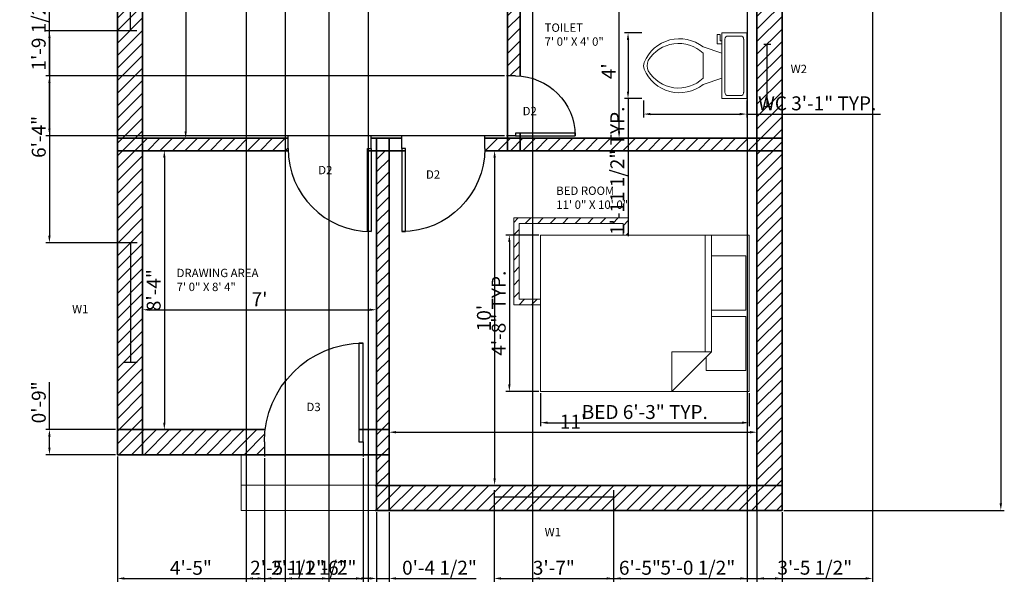
# Model space of a CAD drawing. Units: millimetres. Extents: x 2682 to 3042, y 1647 to 2164.
# Tile 1 of 4: x 2689 to 3042, y 1647 to 1852. Entities that reach past the tile are written whole.
import ezdxf

# ---------------------------------------------------------------- set-up
doc = ezdxf.new("R2010")
doc.units = ezdxf.units.MM
for name, color, linetype, lineweight in [('A-ANNO-TEXT', 170, 'Continuous', 18), ('A-AREA-IDEN', 170, 'Continuous', 18), ('A-FLOR-FIXT', 220, 'Continuous', 18), ('A-WALL-PATT', 3, 'Continuous', 13), ('dimensions', 140, 'Continuous', 18), ('doors', 40, 'Continuous', 25), ('furniture', 220, 'Continuous', 18), ('staircase', 10, 'Continuous', 18), ('walls', 70, 'Continuous', 35), ('windows', 50, 'Continuous', 25)]:
    doc.layers.add(name, color=color, linetype=linetype, lineweight=lineweight)
doc.layers.add('A-FURN-PATT', color=251, linetype='Continuous', lineweight=13, true_color=0x636466)
doc.styles.get("Standard").update_dxf_attribs({"font": 'arial.ttf'})
doc.dimstyles.new('ISO-25', dxfattribs={"dimtxt": 5, "dimasz": 2.5, "dimexe": 1.25, "dimexo": 0.625, "dimtad": 1, "dimdec": 0, "dimlunit": 3, "dimtxsty": 'Standard', "dimcen": 2.5, "dimadec": 0, "dimazin": 0, "dimtfac": 1, "dimtdec": 0, "dimtmove": 0, "dimatfit": 3, "dimfxl": 1, "dimarcsym": 0})

# ---------------------------------------------------------------- blocks, each defined once
blk = doc.blocks.new('*U2')
for p, q in [((0, 0), (0, -6)), ((40, 0), (40, -6))]:
    blk.add_line(p, q)
blk.add_lwpolyline([(0, 0), (0, 40), (1.75, 40), (1.75, 0)], close=True)
blk.add_arc((0, 0), 40, 0, 90)
blk = doc.blocks.new('*U4')
for p, q in [((0, 4), (0, 0)), ((36, 4), (36, 0)), ((0, 2), (36, 2))]:
    blk.add_line(p, q)
blk = doc.blocks.new('*U5')
for p, q in [((0, 4), (0, 0)), ((0, 2), (36, 2)), ((36, 4), (36, 0))]:
    blk.add_line(p, q)
blk = doc.blocks.new('Toilet - top')
for p, q in [((9.5, -6), (9.5, -2)), ((-10, -8.5), (-8, -8.5)), ((-10, -9.5), (-10, -8.5)), ((-8, -8.5), (-8, -8)), ((-7, -8), (-7, -9.5)), ((-4, -8), (-6, -14)), ((4, -8), (6, -14)), ((-7, -9.5), (-10, -9.5)), ((4, -14), (-4, -14))]:
    blk.add_line(p, q)
blk.add_lwpolyline([(10.5, -8), (10.5, 0), (-10.5, 0), (-10.5, -8)], close=True)
for points in [[(-9.5, -2), (-9.5, -6)], [(8.5, -1), (-8.5, -1)], [(-8.5, -7), (8.5, -7)]]:
    blk.add_lwpolyline(points)
for centre, radius, start, end in [((-8.62, -1.88), 0.884, 81.8699, 188.1301), ((8.62, -1.88), 0.884, 351.8699, 98.1301), ((-8.62, -6.12), 0.884, 171.8699, 278.1301), ((8.62, -6.12), 0.884, 261.8699, 8.1301), ((3.52, -21.58), 12.17, 141.4691, 247.9714), ((4.2, -21.82), 11.33, 136.3677, 238.9468), ((-3.52, -21.58), 12.17, 292.0284, 38.5307), ((-4.2, -21.82), 11.33, 301.053, 43.6321), ((0, -27.88), 4, 245.7318, 294.2682), ((0, -29), 4, 254.8605, 285.1395)]:
    blk.add_arc(centre, radius, start, end)
blk = doc.blocks.new('Bed - Queen')
for p, q in [((0, -80.00003), (0, 0)), ((0, 0), (59.99999, 0)), ((59.99999, 0), (59.99999, -80.00003)), ((7.99999, -1.2), (28.79998, -1.2)), ((7.99999, -14.4), (7.99999, -1.2)), ((28.79998, -1.2), (28.79998, -14.4)), ((31.19999, -1.2), (51.99999, -1.2)), ((31.19999, -14.4), (31.19999, -1.2)), ((51.99999, -1.2), (51.99999, -16.4)), ((0, -14.4), (44.8, -14.4)), ((59.99999, -29.6), (44.8, -14.4)), ((44.8, -14.4), (44.8, -29.6)), ((44.8, -16.8), (0, -16.8)), ((51.99999, -16.4), (46.79936, -16.4)), ((44.8, -29.6), (59.99999, -29.6)), ((59.99999, -80.00003), (0, -80.00003))]:
    blk.add_line(p, q)
blk = doc.blocks.new('*D20')
at = {"layer": 'Defpoints', "color": 0, "transparency": 16777216}
for p in [(2903.61, 1857.43), (2911.95, 1857.43), (2911.95, 1809.43)]:
    blk.add_point(p, dxfattribs=at)
at = {"layer": 'dimensions', "color": 0, "lineweight": -2, "transparency": 16777216}
for p, q in [((2911.33, 1857.43), (2902.36, 1857.43)), ((2903.61, 1811.93), (2903.61, 1854.93)), ((2911.33, 1809.43), (2902.36, 1809.43))]:
    blk.add_line(p, q, dxfattribs=at)
at = {"layer": 'dimensions', "color": 0, "transparency": 16777216}
for points in [[(2903.19, 1854.93), (2904.02, 1854.93), (2903.61, 1857.43)], [(2903.19, 1811.93), (2904.02, 1811.93), (2903.61, 1809.43)]]:
    blk.add_solid(points, dxfattribs=at)
at = {"layer": 'dimensions', "color": 0, "transparency": 16777216, "insert": (2900.48, 1833.43), "char_height": 5, "attachment_point": 5, "rotation": 90}
blk.add_mtext("4'", dxfattribs=at)
blk = doc.blocks.new('*D21')
at = {"layer": 'Defpoints', "color": 0, "transparency": 16777216}
for p in [(2953.09, 1703.98), (2821.09, 1700.9), (2953.09, 1700.9)]:
    blk.add_point(p, dxfattribs=at)
at = {"layer": 'dimensions', "color": 0, "lineweight": -2, "transparency": 16777216}
for p, q in [((2821.09, 1701.53), (2821.09, 1705.23)), ((2823.59, 1703.98), (2950.59, 1703.98)), ((2953.09, 1701.53), (2953.09, 1705.23))]:
    blk.add_line(p, q, dxfattribs=at)
at = {"layer": 'dimensions', "color": 0, "transparency": 16777216}
for points in [[(2823.59, 1704.4), (2823.59, 1703.57), (2821.09, 1703.98)], [(2950.59, 1704.4), (2950.59, 1703.57), (2953.09, 1703.98)]]:
    blk.add_solid(points, dxfattribs=at)
at = {"layer": 'dimensions', "color": 0, "transparency": 16777216, "insert": (2887.09, 1707.12), "char_height": 5, "attachment_point": 5}
blk.add_mtext("11'", dxfattribs=at)
blk = doc.blocks.new('*D22')
at = {"layer": 'Defpoints', "color": 0, "transparency": 16777216}
for p in [(2863.59, 1804.93), (2858.95, 1684.93), (2863.59, 1684.93)]:
    blk.add_point(p, dxfattribs=at)
at = {"layer": 'dimensions', "color": 0, "lineweight": -2, "transparency": 16777216}
for p, q in [((2862.96, 1804.93), (2857.7, 1804.93)), ((2858.95, 1802.43), (2858.95, 1687.43)), ((2862.96, 1684.93), (2857.7, 1684.93))]:
    blk.add_line(p, q, dxfattribs=at)
at = {"layer": 'dimensions', "color": 0, "transparency": 16777216}
for points in [[(2858.53, 1802.43), (2859.36, 1802.43), (2858.95, 1804.93)], [(2858.53, 1687.43), (2859.36, 1687.43), (2858.95, 1684.93)]]:
    blk.add_solid(points, dxfattribs=at)
at = {"layer": 'dimensions', "color": 0, "transparency": 16777216, "insert": (2855.77, 1744.93), "char_height": 5, "attachment_point": 5, "rotation": 90}
blk.add_mtext("10'", dxfattribs=at)
blk = doc.blocks.new('*D23')
at = {"layer": 'Defpoints', "color": 0, "transparency": 16777216}
for p in [(2816.59, 1747.9), (2732.59, 1743.81), (2816.59, 1743.81)]:
    blk.add_point(p, dxfattribs=at)
at = {"layer": 'dimensions', "color": 0, "lineweight": -2, "transparency": 16777216}
for p, q in [((2732.59, 1744.44), (2732.59, 1749.15)), ((2816.59, 1744.44), (2816.59, 1749.15)), ((2735.09, 1747.9), (2814.09, 1747.9))]:
    blk.add_line(p, q, dxfattribs=at)
at = {"layer": 'dimensions', "color": 0, "transparency": 16777216}
for points in [[(2735.09, 1748.32), (2735.09, 1747.49), (2732.59, 1747.9)], [(2814.09, 1748.32), (2814.09, 1747.49), (2816.59, 1747.9)]]:
    blk.add_solid(points, dxfattribs=at)
at = {"layer": 'dimensions', "color": 0, "transparency": 16777216, "insert": (2774.59, 1751.03), "char_height": 5, "attachment_point": 5}
blk.add_mtext("7'", dxfattribs=at)
blk = doc.blocks.new('*D24')
at = {"layer": 'Defpoints', "color": 0, "transparency": 16777216}
for p in [(2735.2, 1804.93), (2735.2, 1704.93), (2740.45, 1704.93)]:
    blk.add_point(p, dxfattribs=at)
at = {"layer": 'dimensions', "color": 0, "lineweight": -2, "transparency": 16777216}
for p, q in [((2735.83, 1804.93), (2741.7, 1804.93)), ((2740.45, 1802.43), (2740.45, 1707.43)), ((2735.83, 1704.93), (2741.7, 1704.93))]:
    blk.add_line(p, q, dxfattribs=at)
at = {"layer": 'dimensions', "color": 0, "transparency": 16777216}
for points in [[(2740.03, 1802.43), (2740.87, 1802.43), (2740.45, 1804.93)], [(2740.03, 1707.43), (2740.87, 1707.43), (2740.45, 1704.93)]]:
    blk.add_solid(points, dxfattribs=at)
at = {"layer": 'dimensions', "color": 0, "transparency": 16777216, "insert": (2737.27, 1754.93), "char_height": 5, "attachment_point": 5, "rotation": 90}
blk.add_mtext('8\'-4"', dxfattribs=at)
blk = doc.blocks.new('*D25')
at = {"layer": 'Defpoints', "color": 0, "transparency": 16777216}
for p in [(2751.08, 1998.43), (2748.1, 1809.43), (2751.08, 1809.43)]:
    blk.add_point(p, dxfattribs=at)
at = {"layer": 'dimensions', "color": 0, "lineweight": -2, "transparency": 16777216}
for p, q in [((2750.46, 1998.43), (2746.85, 1998.43)), ((2748.1, 1995.93), (2748.1, 1811.93)), ((2750.46, 1809.43), (2746.85, 1809.43))]:
    blk.add_line(p, q, dxfattribs=at)
at = {"layer": 'dimensions', "color": 0, "transparency": 16777216}
for points in [[(2747.68, 1995.93), (2748.52, 1995.93), (2748.1, 1998.43)], [(2747.68, 1811.93), (2748.52, 1811.93), (2748.1, 1809.43)]]:
    blk.add_solid(points, dxfattribs=at)
at = {"layer": 'dimensions', "color": 0, "transparency": 16777216, "insert": (2744.92, 1903.93), "char_height": 5, "attachment_point": 5, "rotation": 90}
blk.add_mtext('15\'-9"', dxfattribs=at)
blk = doc.blocks.new('*D27')
at = {"layer": 'Defpoints', "color": 0, "transparency": 16777216}
for p in [(2962.09, 2128.93), (2962.09, 1675.93), (3040.59, 1675.93)]:
    blk.add_point(p, dxfattribs=at)
at = {"layer": 'dimensions', "color": 0, "lineweight": -2, "transparency": 16777216}
for p, q in [((2962.71, 2128.93), (3041.84, 2128.93)), ((3040.59, 2126.43), (3040.59, 1678.43)), ((2962.71, 1675.93), (3041.84, 1675.93))]:
    blk.add_line(p, q, dxfattribs=at)
at = {"layer": 'dimensions', "color": 0, "transparency": 16777216}
for points in [[(3040.17, 2126.43), (3041, 2126.43), (3040.59, 2128.93)], [(3040.17, 1678.43), (3041, 1678.43), (3040.59, 1675.93)]]:
    blk.add_solid(points, dxfattribs=at)
at = {"layer": 'dimensions', "color": 0, "transparency": 16777216, "insert": (3037.41, 1902.43), "char_height": 5, "attachment_point": 5, "rotation": 90}
blk.add_mtext("38'", dxfattribs=at)
blk = doc.blocks.new('*D35')
at = {"layer": 'Defpoints', "color": 0, "transparency": 16777216}
for p in [(2875.45, 1718.62), (2950.23, 1718.62), (2950.23, 1707.4)]:
    blk.add_point(p, dxfattribs=at)
at = {"layer": 'dimensions', "color": 0, "lineweight": -2, "transparency": 16777216}
for p, q in [((2875.45, 1717.99), (2875.45, 1706.15)), ((2950.23, 1717.99), (2950.23, 1706.15)), ((2877.95, 1707.4), (2947.73, 1707.4))]:
    blk.add_line(p, q, dxfattribs=at)
at = {"layer": 'dimensions', "color": 0, "transparency": 16777216}
for points in [[(2877.95, 1707.82), (2877.95, 1706.98), (2875.45, 1707.4)], [(2947.73, 1707.82), (2947.73, 1706.98), (2950.23, 1707.4)]]:
    blk.add_solid(points, dxfattribs=at)
at = {"layer": 'dimensions', "color": 0, "transparency": 16777216, "insert": (2912.84, 1710.58), "char_height": 5, "attachment_point": 5}
blk.add_mtext('BED 6\'-3" TYP.', dxfattribs=at)
blk = doc.blocks.new('*D36')
at = {"layer": 'Defpoints', "color": 0, "transparency": 16777216}
for p in [(2875.45, 1774.7), (2864.24, 1718.62), (2875.45, 1718.62)]:
    blk.add_point(p, dxfattribs=at)
at = {"layer": 'dimensions', "color": 0, "lineweight": -2, "transparency": 16777216}
for p, q in [((2874.83, 1774.7), (2862.99, 1774.7)), ((2864.24, 1772.2), (2864.24, 1721.12)), ((2874.83, 1718.62), (2862.99, 1718.62))]:
    blk.add_line(p, q, dxfattribs=at)
at = {"layer": 'dimensions', "color": 0, "transparency": 16777216}
for points in [[(2863.82, 1772.2), (2864.66, 1772.2), (2864.24, 1774.7)], [(2863.82, 1721.12), (2864.66, 1721.12), (2864.24, 1718.62)]]:
    blk.add_solid(points, dxfattribs=at)
at = {"layer": 'dimensions', "color": 0, "transparency": 16777216, "insert": (2861.06, 1746.66), "char_height": 5, "attachment_point": 5, "rotation": 90}
blk.add_mtext('4\'-8" TYP.', dxfattribs=at)
blk = doc.blocks.new('*D37')
at = {"layer": 'Defpoints', "color": 0, "transparency": 16777216}
for p in [(2912.38, 1823.62), (2949.44, 1823.62), (2949.44, 1818.06)]:
    blk.add_point(p, dxfattribs=at)
at = {"layer": 'dimensions', "color": 0, "lineweight": -2, "transparency": 16777216}
for p, q in [((2912.38, 1822.99), (2912.38, 1816.81)), ((2949.44, 1822.99), (2949.44, 1816.81)), ((2914.88, 1818.06), (2946.94, 1818.06)), ((2949.44, 1818.06), (2997.45, 1818.06))]:
    blk.add_line(p, q, dxfattribs=at)
at = {"layer": 'dimensions', "color": 0, "transparency": 16777216}
for points in [[(2914.88, 1818.47), (2914.88, 1817.64), (2912.38, 1818.06)], [(2946.94, 1818.47), (2946.94, 1817.64), (2949.44, 1818.06)]]:
    blk.add_solid(points, dxfattribs=at)
at = {"layer": 'dimensions', "color": 0, "transparency": 16777216, "insert": (2974.7, 1821.27), "char_height": 5, "attachment_point": 5}
blk.add_mtext('WC 3\'-1" TYP.', dxfattribs=at)
blk = doc.blocks.new('*D38')
at = {"layer": 'Defpoints', "color": 0, "transparency": 16777216}
for p in [(2912.38, 1847.17), (2906.83, 1823.62), (2912.38, 1823.62)]:
    blk.add_point(p, dxfattribs=at)
at = {"layer": 'dimensions', "color": 0, "lineweight": -2, "transparency": 16777216}
for p, q in [((2911.76, 1847.17), (2905.58, 1847.17)), ((2906.83, 1844.67), (2906.83, 1826.12)), ((2911.76, 1823.62), (2905.58, 1823.62)), ((2906.83, 1823.62), (2906.83, 1774.32))]:
    blk.add_line(p, q, dxfattribs=at)
at = {"layer": 'dimensions', "color": 0, "transparency": 16777216}
for points in [[(2906.41, 1844.67), (2907.24, 1844.67), (2906.83, 1847.17)], [(2906.41, 1826.12), (2907.24, 1826.12), (2906.83, 1823.62)]]:
    blk.add_solid(points, dxfattribs=at)
at = {"layer": 'dimensions', "color": 0, "transparency": 16777216, "insert": (2903.62, 1797.72), "char_height": 5, "attachment_point": 5, "rotation": 90}
blk.add_mtext('1\'-11 1/2" TYP.', dxfattribs=at)
blk = doc.blocks.new('*D52')
at = {"layer": 'Defpoints', "color": 0, "transparency": 16777216}
for p in [(2769.81, 2100.93), (2799.51, 2100.93), (2799.51, 1651.55)]:
    blk.add_point(p, dxfattribs=at)
at = {"layer": 'dimensions', "color": 0, "lineweight": -2, "transparency": 16777216}
for p, q in [((2769.81, 2100.31), (2769.81, 1650.3)), ((2799.51, 2100.31), (2799.51, 1650.3)), ((2772.31, 1651.55), (2797.01, 1651.55))]:
    blk.add_line(p, q, dxfattribs=at)
at = {"layer": 'dimensions', "color": 0, "transparency": 16777216}
for points in [[(2772.31, 1651.97), (2772.31, 1651.13), (2769.81, 1651.55)], [(2797.01, 1651.97), (2797.01, 1651.13), (2799.51, 1651.55)]]:
    blk.add_solid(points, dxfattribs=at)
at = {"layer": 'dimensions', "color": 0, "transparency": 16777216, "insert": (2784.66, 1654.76), "char_height": 5, "attachment_point": 5}
blk.add_mtext('2\'-5 1/2"', dxfattribs=at)
blk = doc.blocks.new('*D54')
at = {"layer": 'Defpoints', "color": 0, "transparency": 16777216}
for p in [(2872.59, 1909.93), (2949.59, 1909.93), (2949.59, 1651.55)]:
    blk.add_point(p, dxfattribs=at)
at = {"layer": 'dimensions', "color": 0, "lineweight": -2, "transparency": 16777216}
for p, q in [((2872.59, 1909.3), (2872.59, 1650.3)), ((2949.59, 1909.3), (2949.59, 1650.3)), ((2875.09, 1651.55), (2947.09, 1651.55))]:
    blk.add_line(p, q, dxfattribs=at)
at = {"layer": 'dimensions', "color": 0, "transparency": 16777216}
for points in [[(2875.09, 1651.97), (2875.09, 1651.13), (2872.59, 1651.55)], [(2947.09, 1651.97), (2947.09, 1651.13), (2949.59, 1651.55)]]:
    blk.add_solid(points, dxfattribs=at)
at = {"layer": 'dimensions', "color": 0, "transparency": 16777216, "insert": (2911.09, 1654.73), "char_height": 5, "attachment_point": 5}
blk.add_mtext('6\'-5"', dxfattribs=at)
blk = doc.blocks.new('*D55')
at = {"layer": 'Defpoints', "color": 0, "transparency": 16777216}
for p in [(2953.09, 1902.43), (2994.59, 1861.93), (2994.59, 1651.55)]:
    blk.add_point(p, dxfattribs=at)
at = {"layer": 'dimensions', "color": 0, "lineweight": -2, "transparency": 16777216}
for p, q in [((2953.09, 1901.8), (2953.09, 1650.3)), ((2994.59, 1861.3), (2994.59, 1650.3)), ((2955.59, 1651.55), (2992.09, 1651.55))]:
    blk.add_line(p, q, dxfattribs=at)
at = {"layer": 'dimensions', "color": 0, "transparency": 16777216}
for points in [[(2955.59, 1651.97), (2955.59, 1651.13), (2953.09, 1651.55)], [(2992.09, 1651.97), (2992.09, 1651.13), (2994.59, 1651.55)]]:
    blk.add_solid(points, dxfattribs=at)
at = {"layer": 'dimensions', "color": 0, "transparency": 16777216, "insert": (2973.84, 1654.76), "char_height": 5, "attachment_point": 5}
blk.add_mtext('3\'-5 1/2"', dxfattribs=at)
blk = doc.blocks.new('*D56')
at = {"layer": 'Defpoints', "color": 0, "transparency": 16777216}
for p in [(2858.75, 1680.84), (2901.67, 1680.84), (2901.67, 1651.55)]:
    blk.add_point(p, dxfattribs=at)
at = {"layer": 'dimensions', "color": 0, "lineweight": -2, "transparency": 16777216}
for p, q in [((2858.75, 1680.21), (2858.75, 1650.3)), ((2901.67, 1680.21), (2901.67, 1650.3)), ((2861.25, 1651.55), (2899.17, 1651.55))]:
    blk.add_line(p, q, dxfattribs=at)
at = {"layer": 'dimensions', "color": 0, "transparency": 16777216}
for points in [[(2861.25, 1651.97), (2861.25, 1651.13), (2858.75, 1651.55)], [(2899.17, 1651.97), (2899.17, 1651.13), (2901.67, 1651.55)]]:
    blk.add_solid(points, dxfattribs=at)
at = {"layer": 'dimensions', "color": 0, "transparency": 16777216, "insert": (2880.21, 1654.73), "char_height": 5, "attachment_point": 5}
blk.add_mtext('3\'-7"', dxfattribs=at)
blk = doc.blocks.new('*D59')
at = {"layer": 'Defpoints', "color": 0, "transparency": 16777216}
for p in [(2783.8, 1996.99), (2813.59, 1996.99), (2813.59, 1651.55)]:
    blk.add_point(p, dxfattribs=at)
at = {"layer": 'dimensions', "color": 0, "lineweight": -2, "transparency": 16777216}
for p, q in [((2783.8, 1996.36), (2783.8, 1650.3)), ((2813.59, 1996.36), (2813.59, 1650.3)), ((2786.3, 1651.55), (2811.09, 1651.55))]:
    blk.add_line(p, q, dxfattribs=at)
at = {"layer": 'dimensions', "color": 0, "transparency": 16777216}
for points in [[(2786.3, 1651.97), (2786.3, 1651.13), (2783.8, 1651.55)], [(2811.09, 1651.97), (2811.09, 1651.13), (2813.59, 1651.55)]]:
    blk.add_solid(points, dxfattribs=at)
at = {"layer": 'dimensions', "color": 0, "transparency": 16777216, "insert": (2798.69, 1654.73), "char_height": 5, "attachment_point": 5}
blk.add_mtext('2\'-6"', dxfattribs=at)
blk = doc.blocks.new('*D60')
at = {"layer": 'Defpoints', "color": 0, "transparency": 16777216}
for p in [(2699.21, 1831.73), (2863.18, 1831.73), (2863.18, 1810.31)]:
    blk.add_point(p, dxfattribs=at)
at = {"layer": 'dimensions', "color": 0, "lineweight": -2, "transparency": 16777216}
for p, q in [((2699.21, 1831.73), (2699.21, 1859.95)), ((2862.55, 1831.73), (2697.96, 1831.73)), ((2699.21, 1812.81), (2699.21, 1829.23)), ((2862.55, 1810.31), (2697.96, 1810.31))]:
    blk.add_line(p, q, dxfattribs=at)
at = {"layer": 'dimensions', "color": 0, "transparency": 16777216}
for points in [[(2698.8, 1829.23), (2699.63, 1829.23), (2699.21, 1831.73)], [(2698.8, 1812.81), (2699.63, 1812.81), (2699.21, 1810.31)]]:
    blk.add_solid(points, dxfattribs=at)
at = {"layer": 'dimensions', "color": 0, "transparency": 16777216, "insert": (2696, 1847.09), "char_height": 5, "attachment_point": 5, "rotation": 90}
blk.add_mtext('1\'-9 1/2"', dxfattribs=at)
blk = doc.blocks.new('*D61')
at = {"layer": 'Defpoints', "color": 0, "transparency": 16777216}
for p in [(2776.38, 1695.25), (2811.76, 1695.25), (2811.76, 1651.55)]:
    blk.add_point(p, dxfattribs=at)
at = {"layer": 'dimensions', "color": 0, "lineweight": -2, "transparency": 16777216}
for p, q in [((2776.38, 1694.63), (2776.38, 1650.3)), ((2811.76, 1694.63), (2811.76, 1650.3)), ((2778.88, 1651.55), (2809.26, 1651.55))]:
    blk.add_line(p, q, dxfattribs=at)
at = {"layer": 'dimensions', "color": 0, "transparency": 16777216}
for points in [[(2778.88, 1651.97), (2778.88, 1651.13), (2776.38, 1651.55)], [(2809.26, 1651.97), (2809.26, 1651.13), (2811.76, 1651.55)]]:
    blk.add_solid(points, dxfattribs=at)
at = {"layer": 'dimensions', "color": 0, "transparency": 16777216, "insert": (2794.07, 1654.76), "char_height": 5, "attachment_point": 5}
blk.add_mtext('2\'-11 1/2"', dxfattribs=at)
blk = doc.blocks.new('*D62')
at = {"layer": 'Defpoints', "color": 0, "transparency": 16777216}
for p in [(2723.59, 1695.93), (2776.38, 1695.25), (2776.38, 1651.55)]:
    blk.add_point(p, dxfattribs=at)
at = {"layer": 'dimensions', "color": 0, "lineweight": -2, "transparency": 16777216}
for p, q in [((2723.59, 1695.3), (2723.59, 1650.3)), ((2776.38, 1694.63), (2776.38, 1650.3)), ((2726.09, 1651.55), (2773.88, 1651.55))]:
    blk.add_line(p, q, dxfattribs=at)
at = {"layer": 'dimensions', "color": 0, "transparency": 16777216}
for points in [[(2726.09, 1651.97), (2726.09, 1651.13), (2723.59, 1651.55)], [(2773.88, 1651.97), (2773.88, 1651.13), (2776.38, 1651.55)]]:
    blk.add_solid(points, dxfattribs=at)
at = {"layer": 'dimensions', "color": 0, "transparency": 16777216, "insert": (2749.98, 1654.72), "char_height": 5, "attachment_point": 5}
blk.add_mtext('4\'-5"', dxfattribs=at)
blk = doc.blocks.new('*D63')
at = {"layer": 'Defpoints', "color": 0, "transparency": 16777216}
for p in [(2699.21, 1704.93), (2723.59, 1704.93), (2723.59, 1695.93)]:
    blk.add_point(p, dxfattribs=at)
at = {"layer": 'dimensions', "color": 0, "lineweight": -2, "transparency": 16777216}
for p, q in [((2699.21, 1704.93), (2699.21, 1721.97)), ((2722.96, 1704.93), (2697.96, 1704.93)), ((2699.21, 1698.43), (2699.21, 1702.43)), ((2722.96, 1695.93), (2697.96, 1695.93))]:
    blk.add_line(p, q, dxfattribs=at)
at = {"layer": 'dimensions', "color": 0, "transparency": 16777216}
for points in [[(2698.8, 1702.43), (2699.63, 1702.43), (2699.21, 1704.93)], [(2698.8, 1698.43), (2699.63, 1698.43), (2699.21, 1695.93)]]:
    blk.add_solid(points, dxfattribs=at)
at = {"layer": 'dimensions', "color": 0, "transparency": 16777216, "insert": (2696.03, 1714.7), "char_height": 5, "attachment_point": 5, "rotation": 90}
blk.add_mtext('0\'-9"', dxfattribs=at)
blk = doc.blocks.new('*D64')
at = {"layer": 'Defpoints', "color": 0, "transparency": 16777216}
for p in [(2816.59, 1675.93), (2821.09, 1675.93), (2821.09, 1651.55)]:
    blk.add_point(p, dxfattribs=at)
at = {"layer": 'dimensions', "color": 0, "lineweight": -2, "transparency": 16777216}
for p, q in [((2816.59, 1675.3), (2816.59, 1650.3)), ((2821.09, 1675.3), (2821.09, 1650.3)), ((2814.09, 1651.55), (2811.59, 1651.55)), ((2816.59, 1651.55), (2821.09, 1651.55)), ((2823.59, 1651.55), (2852.28, 1651.55))]:
    blk.add_line(p, q, dxfattribs=at)
at = {"layer": 'dimensions', "color": 0, "transparency": 16777216}
for points in [[(2814.09, 1651.97), (2814.09, 1651.13), (2816.59, 1651.55)], [(2823.59, 1651.97), (2823.59, 1651.13), (2821.09, 1651.55)]]:
    blk.add_solid(points, dxfattribs=at)
at = {"layer": 'dimensions', "color": 0, "transparency": 16777216, "insert": (2839.18, 1654.76), "char_height": 5, "attachment_point": 5}
blk.add_mtext('0\'-4 1/2"', dxfattribs=at)
blk = doc.blocks.new('*D70')
at = {"layer": 'Defpoints', "color": 0, "transparency": 16777216}
for p in [(2728.2, 1847.86), (2699.21, 1771.91), (2728.36, 1771.91)]:
    blk.add_point(p, dxfattribs=at)
at = {"layer": 'dimensions', "color": 0, "lineweight": -2, "transparency": 16777216}
for p, q in [((2727.58, 1847.86), (2697.96, 1847.86)), ((2699.21, 1845.36), (2699.21, 1774.41)), ((2727.73, 1771.91), (2697.96, 1771.91))]:
    blk.add_line(p, q, dxfattribs=at)
at = {"layer": 'dimensions', "color": 0, "transparency": 16777216}
for points in [[(2698.8, 1845.36), (2699.63, 1845.36), (2699.21, 1847.86)], [(2698.8, 1774.41), (2699.63, 1774.41), (2699.21, 1771.91)]]:
    blk.add_solid(points, dxfattribs=at)
at = {"layer": 'dimensions', "color": 0, "transparency": 16777216, "insert": (2696.03, 1809.88), "char_height": 5, "attachment_point": 5, "rotation": 90}
blk.add_mtext('6\'-4"', dxfattribs=at)
blk = doc.blocks.new('*D71')
at = {"layer": 'Defpoints', "color": 0, "transparency": 16777216}
for p in [(2901.67, 1680.84), (2962.09, 1675.93), (2962.09, 1651.55)]:
    blk.add_point(p, dxfattribs=at)
at = {"layer": 'dimensions', "color": 0, "lineweight": -2, "transparency": 16777216}
for p, q in [((2901.67, 1680.21), (2901.67, 1650.3)), ((2962.09, 1675.3), (2962.09, 1650.3)), ((2904.17, 1651.55), (2959.59, 1651.55))]:
    blk.add_line(p, q, dxfattribs=at)
at = {"layer": 'dimensions', "color": 0, "transparency": 16777216}
for points in [[(2904.17, 1651.97), (2904.17, 1651.13), (2901.67, 1651.55)], [(2959.59, 1651.97), (2959.59, 1651.13), (2962.09, 1651.55)]]:
    blk.add_solid(points, dxfattribs=at)
at = {"layer": 'dimensions', "color": 0, "transparency": 16777216, "insert": (2931.88, 1654.76), "char_height": 5, "attachment_point": 5}
blk.add_mtext('5\'-0 1/2"', dxfattribs=at)

msp = doc.modelspace()

# ---------------------------------------------------------------- hatches: boundary and pattern name
at = {"layer": 'A-FURN-PATT'}
h = msp.add_hatch(dxfattribs=at)
h.set_pattern_fill('ANSI31', color=256)
h.paths.add_polyline_path([(2868.36, 2054.1), (2875.35, 2054.1), (2875.35, 2056.1), (2866.36, 2056.1), (2866.36, 2017.68), (2900.8, 2017.68), (2900.8, 2036.29), (2898.8, 2036.29), (2898.8, 2019.68), (2868.36, 2019.68)])
h.paths.add_polyline_path([(2907.02, 1780.81), (2865.81, 1780.81), (2865.81, 1749.67), (2875.45, 1749.67), (2875.45, 1751.67), (2867.81, 1751.67), (2867.81, 1778.81), (2905.02, 1778.81), (2905.02, 1774.7), (2907.02, 1774.7)])
at = {"layer": 'A-WALL-PATT'}
h = msp.add_hatch(dxfattribs=at)
h.set_pattern_fill('ANSI31', color=256)
h.paths.add_polyline_path([(2816.59, 2128.93), (2732.59, 2128.93), (2732.59, 2119.93), (2816.59, 2119.93)])
h.paths.add_polyline_path([(2953.09, 2128.93), (2821.09, 2128.93), (2821.09, 2119.93), (2953.09, 2119.93)])
h.paths.add_polyline_path([(2821.09, 2119.93), (2816.59, 2119.93), (2816.59, 2002.93), (2821.09, 2002.93)])
h.paths.add_polyline_path([(2821.09, 2128.93), (2816.59, 2128.93), (2816.59, 2119.93), (2821.09, 2119.93)])
h.paths.add_polyline_path([(2732.59, 2119.93), (2723.59, 2119.93), (2723.59, 2002.93), (2732.59, 2002.93)])
h.paths.add_polyline_path([(2732.59, 2128.93), (2723.59, 2128.93), (2723.59, 2119.93), (2732.59, 2119.93)])
h.paths.add_polyline_path([(2962.09, 2119.93), (2953.09, 2119.93), (2953.09, 2002.93), (2962.09, 2002.93)])
h.paths.add_polyline_path([(2962.09, 2128.93), (2953.09, 2128.93), (2953.09, 2119.93), (2962.09, 2119.93)])
h.paths.add_polyline_path([(2953.09, 2002.93), (2897.45, 2002.93), (2897.45, 2000.43, -0.023466), (2897.35, 1998.43), (2953.09, 1998.43)])
h.paths.add_polyline_path([(2962.09, 1998.43), (2953.09, 1998.43), (2953.09, 1950.43), (2962.09, 1950.43)])
h.paths.add_polyline_path([(2953.09, 1950.43), (2868.09, 1950.43), (2868.09, 1945.93), (2953.09, 1945.93)])
h.paths.add_polyline_path([(2994.59, 1950.43), (2962.09, 1950.43), (2962.09, 1945.93), (2994.59, 1945.93)])
h.paths.add_polyline_path([(2868.09, 1998.43), (2863.59, 1998.43), (2863.59, 1950.43), (2868.09, 1950.43)])
h.paths.add_polyline_path([(2868.09, 2002.93), (2863.59, 2002.93), (2863.59, 1998.43), (2868.09, 1998.43)])
h.paths.add_polyline_path([(2863.59, 2002.93), (2853.46, 2002.93, -0.011786), (2853.49, 2001.52), (2853.49, 1998.43), (2863.59, 1998.43)])
h.paths.add_polyline_path([(2783.8, 2001.45, -0.012351), (2783.84, 2002.93), (2756.59, 2002.93), (2756.59, 2002.69), (2732.59, 2002.93), (2732.59, 1998.43), (2783.8, 1998.43)])
h.paths.add_polyline_path([(2732.59, 2002.93), (2723.59, 2002.93), (2723.59, 1998.43), (2732.59, 1998.43)])
h.paths.add_polyline_path([(2732.59, 1998.43), (2723.59, 1998.43), (2723.59, 1809.43), (2732.59, 1809.43)])
h.paths.add_polyline_path([(2994.59, 1861.93), (2962.09, 1861.93), (2962.09, 1857.43), (2994.59, 1857.43)])
h.paths.add_polyline_path([(2999.09, 1884.37), (2994.59, 1884.37), (2994.59, 1861.93), (2999.09, 1861.93)])
h.paths.add_polyline_path([(2953.09, 1861.93), (2868.09, 1861.93), (2868.09, 1857.43), (2953.09, 1857.43)])
h.paths.add_polyline_path([(2962.09, 1861.93), (2953.09, 1861.93), (2953.09, 1857.43), (2962.09, 1857.43)])
h.paths.add_polyline_path([(2868.09, 1857.43), (2863.59, 1857.43), (2863.59, 1831.73), (2866.39, 1831.73, -0.019816), (2868.09, 1831.66)])
h.paths.add_polyline_path([(2868.09, 1861.93), (2863.59, 1861.93), (2863.59, 1857.43), (2868.09, 1857.43)])
h.paths.add_polyline_path([(2962.09, 1804.93), (2953.09, 1804.93), (2953.09, 1684.93), (2962.09, 1684.93)])
h.paths.add_polyline_path([(2962.09, 1857.43), (2953.09, 1857.43), (2953.09, 1809.43), (2962.09, 1809.43)])
h.paths.add_polyline_path([(2962.09, 1809.43), (2953.09, 1809.43), (2953.09, 1804.93), (2962.09, 1804.93)])
h.paths.add_polyline_path([(2953.09, 1809.43), (2868.09, 1809.43), (2868.09, 1804.93), (2953.09, 1804.93)])
h.paths.add_polyline_path([(2868.09, 1809.43), (2863.59, 1809.43), (2863.59, 1804.93), (2868.09, 1804.93)])
h.paths.add_polyline_path([(2863.59, 1809.43), (2855.42, 1809.43), (2855.42, 1805.73, -0.006742), (2855.41, 1804.93), (2863.59, 1804.93)])
h.paths.add_polyline_path([(2953.09, 1684.93), (2863.59, 1684.93), (2821.09, 1684.93), (2821.09, 1675.93), (2863.59, 1675.93), (2953.09, 1675.93)])
h.paths.add_polyline_path([(2962.09, 1684.93), (2953.09, 1684.93), (2953.09, 1675.93), (2962.09, 1675.93)])
h.paths.add_polyline_path([(2821.09, 1804.93), (2816.59, 1804.93), (2816.59, 1704.93), (2821.09, 1704.93)])
h.paths.add_polyline_path([(2821.09, 1695.93), (2816.59, 1695.93), (2816.59, 1684.93), (2821.09, 1684.93)])
h.paths.add_polyline_path([(2821.09, 1704.93), (2816.59, 1704.93), (2816.59, 1695.93), (2821.09, 1695.93)])
h.paths.add_polyline_path([(2821.09, 1684.93), (2816.59, 1684.93), (2816.59, 1675.93), (2821.09, 1675.93)])
h.paths.add_polyline_path([(2776.38, 1700.56, -0.030957), (2776.65, 1704.93), (2732.59, 1704.93), (2732.59, 1695.93), (2776.38, 1695.93)])
h.paths.add_polyline_path([(2732.59, 1804.93), (2723.59, 1804.93), (2723.59, 1704.93), (2732.59, 1704.93)])
h.paths.add_polyline_path([(2732.59, 1704.93), (2723.59, 1704.93), (2723.59, 1695.93), (2732.59, 1695.93)])
h.paths.add_polyline_path([(2999.09, 1945.93), (2994.59, 1945.93), (2994.59, 1937.59), (2999.09, 1937.59)])
h.paths.add_polyline_path([(2999.09, 1937.59), (2996.77, 1937.59), (2996.77, 1884.37), (2999.09, 1884.37)])
h.paths.add_polyline_path([(2996.77, 1937.59), (2994.59, 1937.59), (2994.59, 1884.37), (2996.77, 1884.37)])
h.paths.add_polyline_path([(2784.83, 1809.43), (2732.59, 1809.43), (2732.59, 1804.93), (2784.84, 1804.93, -0.006742), (2784.83, 1805.73)])
h.paths.add_polyline_path([(2732.59, 1809.43), (2723.59, 1809.43), (2723.59, 1804.93), (2732.59, 1804.93)])

# ---------------------------------------------------------------- linework, layer by layer
at = {"layer": 'furniture'}
for points in [[(2875.45, 1749.67), (2865.81, 1749.67), (2865.81, 1780.81), (2907.02, 1780.81), (2907.02, 1774.7)], [(2875.45, 1751.67), (2867.81, 1751.67), (2867.81, 1778.81), (2905.02, 1778.81), (2905.02, 1774.7)]]:
    msp.add_lwpolyline(points, dxfattribs=at)
at = {"layer": 'staircase'}
for p, q in [((2768.01, 1695.93), (2768.01, 1684.96)), ((2768.01, 1684.96), (2816.59, 1684.96)), ((2768.01, 1684.96), (2768.01, 1678.16)), ((2768.01, 1675.93), (2768.01, 1678.16)), ((2768.01, 1675.93), (2816.59, 1675.93)), ((2816.59, 1675.93), (2768.01, 1675.93))]:
    msp.add_line(p, q, dxfattribs=at)
at = {"layer": 'walls'}
for p, q in [((2723.59, 2128.93), (2723.59, 1695.93)), ((2732.59, 2128.93), (2732.59, 1695.93)), ((2953.09, 2128.93), (2953.09, 1675.93)), ((2863.59, 1861.93), (2863.59, 1804.93)), ((2868.09, 1861.93), (2868.09, 1831.66)), ((2962.09, 1861.93), (2962.09, 1675.93)), ((2723.59, 1809.43), (2784.83, 1809.43)), ((2814.62, 1809.43), (2825.64, 1809.43)), ((2816.59, 1809.43), (2816.59, 1675.93)), ((2821.09, 1809.43), (2821.09, 1695.93)), ((2821.09, 1809.43), (2821.09, 1675.93)), ((2855.42, 1809.43), (2868.09, 1809.43)), ((2863.59, 1809.43), (2962.09, 1809.43)), ((2868.09, 1811.25), (2868.09, 1804.93)), ((2723.59, 1804.93), (2784.84, 1804.93)), ((2813.32, 1804.93), (2826.94, 1804.93)), ((2855.41, 1804.93), (2868.09, 1804.93)), ((2863.59, 1804.93), (2962.09, 1804.93)), ((2723.59, 1704.93), (2776.65, 1704.93)), ((2810.21, 1704.93), (2821.09, 1704.93)), ((2723.59, 1695.93), (2821.09, 1695.93)), ((2863.59, 1684.93), (2816.06, 1684.93)), ((2863.59, 1684.93), (2962.09, 1684.93)), ((2863.59, 1675.93), (2816.06, 1675.93)), ((2863.59, 1675.93), (2962.09, 1675.93))]:
    msp.add_line(p, q, dxfattribs=at)

# ---------------------------------------------------------------- block references
at = {"layer": 'A-FLOR-FIXT', "xscale": 1.121371250506495, "yscale": 1.121371250506495, "zscale": 1.121371250506495, "rotation": 269.9999999999973}
msp.add_blockref('Toilet - top', (2949.44, 1835.39), dxfattribs=at)
at = {"layer": 'doors'}
for p, xscale, yscale, zscale, rotation in [((2866.39, 1810.31), -0.5354065160128529, 0.5354065160128529, 0.5354065160128529, 270), ((2814.62, 1805.73), 0.744697270728857, 0.744697270728857, 0.744697270728857, 180), ((2825.64, 1805.73), -0.744697270728857, 0.744697270728857, 0.744697270728857, 180)]:
    msp.add_blockref('*U2', p, dxfattribs=dict(at, xscale=xscale, yscale=yscale, zscale=zscale, rotation=rotation))
at = {"layer": 'doors', "xscale": -0.8844760457410782, "yscale": 0.8844760457410782, "zscale": 0.8844760457410782}
msp.add_blockref('*U2', (2811.76, 1700.56), dxfattribs=at)
at = {"layer": 'furniture', "xscale": 0.9346925861226617, "yscale": 0.9346925861226617, "zscale": 0.9346925861226617, "rotation": 269.9999999999884}
msp.add_blockref('Bed - Queen', (2950.23, 1774.7), dxfattribs=at)
at = {"layer": 'windows'}
for name, p, xscale, yscale, zscale, rotation in [('*U4', (2725.82, 1890.78), 1.192221816707046, 1.192221816707046, 1.192221816707046, 270), ('*U5', (2958.03, 1820.84), 0.6208711624712905, 0.6208711624712905, 0.6208711624712905, 90), ('*U4', (2725.97, 1771.91), 1.192221816707046, 1.192221816707046, 1.192221816707046, 270)]:
    msp.add_blockref(name, p, dxfattribs=dict(at, xscale=xscale, yscale=yscale, zscale=zscale, rotation=rotation))
at = {"layer": 'windows', "xscale": 1.192221816707046, "yscale": 1.192221816707046, "zscale": 1.192221816707046}
msp.add_blockref('*U4', (2858.75, 1678.45), dxfattribs=at)

# ---------------------------------------------------------------- texts
at = {"layer": 'A-ANNO-TEXT', "char_height": 3, "attachment_point": 1}
for s, width, insert in [('W2', 17.3612, (2965.17, 1835.74)), ('D2', 10.4757, (2869.01, 1820.65)), ('D2', 15.5328, (2795.66, 1799.48)), ('D2', 14.1591, (2834.33, 1797.89)), ('W1', 12.3833, (2707.35, 1749.66)), ('D3', 15.4098, (2791.46, 1714.55)), ('W1', 13.8484, (2876.9, 1669.69))]:
    msp.add_mtext_dynamic_manual_height_columns(s, width=width, gutter_width=12.5, heights=[0], dxfattribs=dict(at, insert=insert))
at = {"layer": 'A-AREA-IDEN', "char_height": 3, "attachment_point": 1}
for s, width, insert in [('TOILET\\P7\' 0" X 4\' 0"', 39.5175, (2876.89, 1850.56)), ('BED ROOM \\P11\' 0" X 10\' 0"', 47.2752, (2881.07, 1792.08)), ('DRAWING AREA \\P7\' 0" X 8\' 4"', 55.9803, (2744.85, 1762.59))]:
    msp.add_mtext_dynamic_manual_height_columns(s, width=width, gutter_width=12.5, heights=[0], dxfattribs=dict(at, insert=insert))

# ---------------------------------------------------------------- dimensions: what is measured, and where the dimension line sits
at = {"layer": 'dimensions'}
for base, p1, p2, angle, text, override, picture, middle in [((3040.59, 1675.93), (2962.09, 2128.93), (2962.09, 1675.93), 90, "38'", {"dimclrd": 0, "dimclre": 0, "dimclrt": 0}, '*D27', (3037.41, 1902.43)), ((2906.8264, 1823.6167), (2912.385, 1847.1655), (2912.385, 1823.6167), 270, '<> TYP.', {"dimdec": 1, "dimlfac": 1, "dimrnd": 0, "dimzin": 1, "dimdsep": 46, "dimlunit": 4, "dimfrac": 2}, '*D38', (2903.6162, 1797.7206)), ((2864.24, 1718.62), (2875.45, 1774.7), (2875.45, 1718.62), 270, '<> TYP.', {"dimdec": 1, "dimlfac": 1, "dimrnd": 0, "dimzin": 1, "dimdsep": 46, "dimlunit": 4, "dimfrac": 2}, '*D36', (2861.06, 1746.66))]:
    dim = msp.add_linear_dim(base=base, p1=p1, p2=p2, angle=angle, text=text, dimstyle='ISO-25', override=override, dxfattribs=at)
    dim.commit()
    dim.dimension.update_dxf_attribs({"geometry": picture, "text_midpoint": middle})
for base, p1, p2, override, picture, middle in [((2799.51, 1651.55), (2769.81, 2100.93), (2799.51, 2100.93), {"dimdec": 1, "dimlfac": 1, "dimrnd": 0, "dimzin": 1, "dimdsep": 46, "dimlunit": 4, "dimfrac": 2}, '*D52', (2784.66, 1654.76)), ((2813.59, 1651.55), (2783.8, 1996.99), (2813.59, 1996.99), {"dimdec": 1, "dimlfac": 1, "dimrnd": 0, "dimzin": 1, "dimdsep": 46, "dimlunit": 4, "dimfrac": 2}, '*D59', (2798.69, 1654.73)), ((2949.59, 1651.55), (2872.59, 1909.93), (2949.59, 1909.93), {"dimdec": 1, "dimlfac": 1, "dimrnd": 0, "dimzin": 1, "dimdsep": 46, "dimlunit": 4, "dimfrac": 2}, '*D54', (2911.09, 1654.73)), ((2994.59, 1651.55), (2953.09, 1902.43), (2994.59, 1861.93), {"dimdec": 1, "dimlfac": 1, "dimrnd": 0, "dimzin": 1, "dimdsep": 46, "dimlunit": 4, "dimfrac": 2}, '*D55', (2973.84, 1654.76)), ((2816.59, 1747.9), (2732.59, 1743.81), (2816.59, 1743.81), {"dimclrd": 0, "dimclre": 0, "dimclrt": 0}, '*D23', (2774.59, 1751.03)), ((2953.09, 1703.98), (2821.09, 1700.9), (2953.09, 1700.9), {"dimclrd": 0, "dimclre": 0, "dimclrt": 0}, '*D21', (2887.09, 1707.12)), ((2776.38, 1651.55), (2723.59, 1695.93), (2776.38, 1695.25), {"dimdec": 1, "dimlfac": 1, "dimrnd": 0, "dimzin": 1, "dimdsep": 46, "dimlunit": 4, "dimfrac": 2}, '*D62', (2749.98, 1654.72)), ((2811.76, 1651.55), (2776.38, 1695.25), (2811.76, 1695.25), {"dimdec": 1, "dimlfac": 1, "dimrnd": 0, "dimzin": 1, "dimdsep": 46, "dimlunit": 4, "dimfrac": 2}, '*D61', (2794.07, 1654.76)), ((2901.67, 1651.55), (2858.75, 1680.84), (2901.67, 1680.84), {"dimdec": 1, "dimlfac": 1, "dimrnd": 0, "dimzin": 1, "dimdsep": 46, "dimlunit": 4, "dimfrac": 2}, '*D56', (2880.21, 1654.73)), ((2962.09, 1651.55), (2901.67, 1680.84), (2962.09, 1675.93), {"dimdec": 1, "dimlfac": 1, "dimrnd": 0, "dimzin": 1, "dimdsep": 46, "dimlunit": 4, "dimfrac": 2}, '*D71', (2931.88, 1654.76)), ((2821.09, 1651.55), (2816.59, 1675.93), (2821.09, 1675.93), {"dimdec": 1, "dimlfac": 1, "dimrnd": 0, "dimzin": 1, "dimdsep": 46, "dimlunit": 4, "dimfrac": 2}, '*D64', (2839.18, 1654.76))]:
    dim = msp.add_linear_dim(base=base, p1=p1, p2=p2, dimstyle='ISO-25', override=override, dxfattribs=at)
    dim.commit()
    dim.dimension.update_dxf_attribs({"geometry": picture, "text_midpoint": middle})
for base, p1, p2, override, picture, middle in [((2748.1, 1809.43), (2751.08, 1998.43), (2751.08, 1809.43), {"dimclrd": 0, "dimclre": 0, "dimclrt": 0}, '*D25', (2744.92, 1903.93)), ((2699.21, 1831.73), (2863.18, 1810.31), (2863.18, 1831.73), {"dimdec": 1, "dimlfac": 1, "dimrnd": 0, "dimzin": 1, "dimdsep": 46, "dimlunit": 4, "dimfrac": 2}, '*D60', (2696, 1847.09)), ((2903.61, 1857.43), (2911.95, 1809.43), (2911.95, 1857.43), {"dimclrd": 0, "dimclre": 0, "dimclrt": 0}, '*D20', (2900.48, 1833.43)), ((2699.2122, 1771.9108), (2728.2018, 1847.8588), (2728.3561, 1771.9108), {"dimdec": 1, "dimlfac": 1, "dimrnd": 0, "dimzin": 1, "dimdsep": 46, "dimlunit": 4, "dimfrac": 2}, '*D70', (2696.0343, 1809.8848)), ((2740.45, 1704.93), (2735.2, 1804.93), (2735.2, 1704.93), {"dimclrd": 0, "dimclre": 0, "dimclrt": 0}, '*D24', (2737.27, 1754.93)), ((2858.95, 1684.93), (2863.59, 1804.93), (2863.59, 1684.93), {"dimclrd": 0, "dimclre": 0, "dimclrt": 0}, '*D22', (2855.77, 1744.93)), ((2699.21, 1704.93), (2723.59, 1695.93), (2723.59, 1704.93), {"dimdec": 1, "dimlfac": 1, "dimrnd": 0, "dimzin": 1, "dimdsep": 46, "dimlunit": 4, "dimfrac": 2}, '*D63', (2696.03, 1714.7))]:
    dim = msp.add_linear_dim(base=base, p1=p1, p2=p2, angle=90, dimstyle='ISO-25', override=override, dxfattribs=at)
    dim.commit()
    dim.dimension.update_dxf_attribs({"geometry": picture, "text_midpoint": middle})
for base, p1, p2, text, picture, middle in [((2949.44, 1818.06), (2912.38, 1823.62), (2949.44, 1823.62), 'WC <> TYP.', '*D37', (2974.7, 1821.27)), ((2950.23, 1707.4), (2875.45, 1718.62), (2950.23, 1718.62), 'BED <> TYP.', '*D35', (2912.84, 1710.58))]:
    dim = msp.add_linear_dim(base=base, p1=p1, p2=p2, text=text, dimstyle='ISO-25', override={"dimdec": 1, "dimlfac": 1, "dimrnd": 0, "dimzin": 1, "dimdsep": 46, "dimlunit": 4, "dimfrac": 2}, dxfattribs=at)
    dim.commit()
    dim.dimension.update_dxf_attribs({"geometry": picture, "text_midpoint": middle})

doc.saveas('drawing.dxf')
